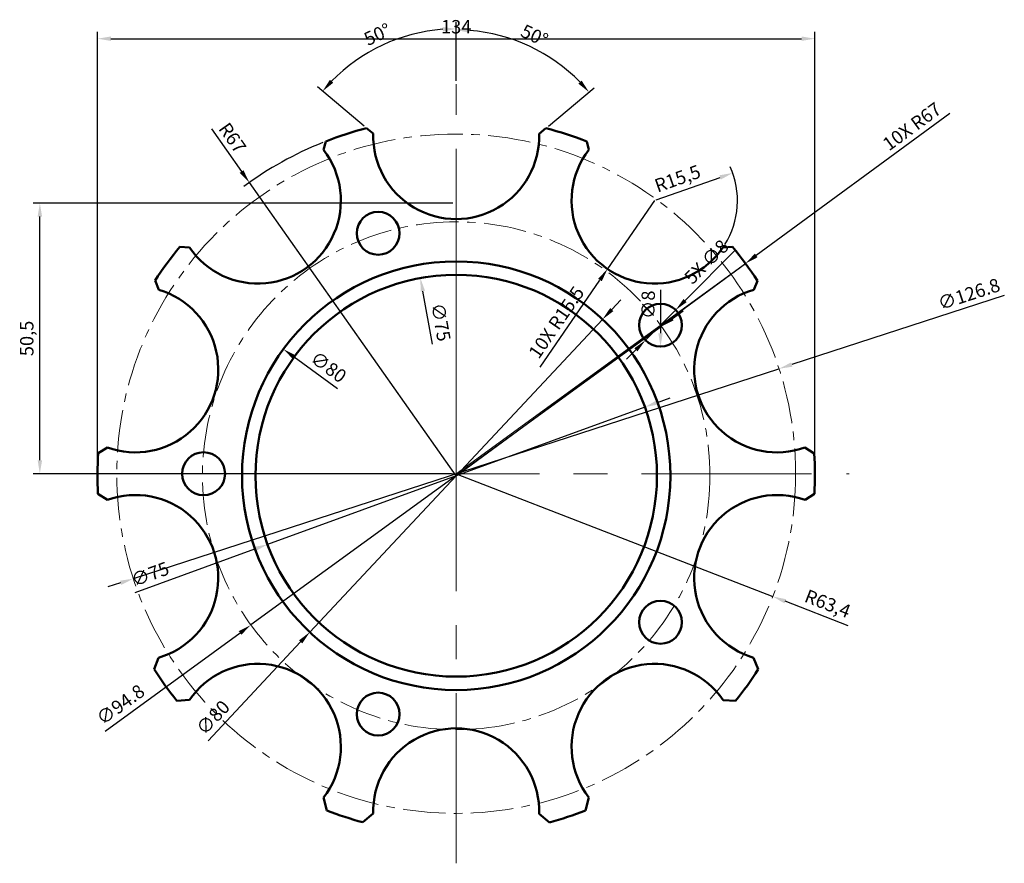
# Model space of a CAD drawing. Units: millimetres. Extents: x 3156 to 3340, y 1440 to 1598.
import ezdxf

# ---------------------------------------------------------------- set-up
doc = ezdxf.new("R2010")
doc.units = ezdxf.units.MM
doc.linetypes.add('CENTER', pattern=[50.8, 31.75, -6.35, 6.35, -6.35])
for name, color, linetype, lineweight in [('M-CNTR', 4, 'CENTER', 18), ('M-CONS', 8, 'Continuous', 13), ('M-DIMS', 2, 'Continuous', 25), ('M-OUTL', 7, 'Continuous', 50)]:
    doc.layers.add(name, color=color, linetype=linetype, lineweight=lineweight)
doc.styles.get("Standard").update_dxf_attribs({"font": 'arial.ttf'})
doc.dimstyles.new('ISO-25', dxfattribs={"dimtxt": 2.5, "dimasz": 2.5, "dimexe": 1.25, "dimexo": 0.625, "dimtad": 1, "dimtxsty": 'Standard', "dimcen": 2.5, "dimadec": 0, "dimazin": 0, "dimtfac": 1, "dimtmove": 0, "dimatfit": 3, "dimfxl": 1, "dimarcsym": 0})

# ---------------------------------------------------------------- blocks, each defined once
blk = doc.blocks.new('*D1')
at = {"layer": 'Defpoints', "color": 0, "transparency": 16777216}
for p in [(3289.21, 1569.14), (3274.59, 1563.99)]:
    blk.add_point(p, dxfattribs=at)
at = {"layer": 'M-DIMS', "color": 0, "lineweight": -2, "transparency": 16777216}
blk.add_line((3274.92, 1564.1), (3286.85, 1568.3), dxfattribs=at)
blk.add_arc((3274.59, 1563.99), 15.5, 327.9019, 24.0231, dxfattribs=at)
at = {"layer": 'M-DIMS', "color": 0, "transparency": 16777216}
blk.add_solid([(3286.71, 1568.7), (3286.99, 1567.91), (3289.21, 1569.14)], dxfattribs=at)
at = {"layer": 'M-DIMS', "color": 0, "transparency": 16777216, "insert": (3279, 1567.79), "char_height": 2.5, "attachment_point": 5, "rotation": 19.4025}
blk.add_mtext('R15,5', dxfattribs=at)
blk = doc.blocks.new('*D2')
at = {"layer": 'Defpoints', "color": 0, "transparency": 16777216}
for p in [(3198.91, 1567.36), (3237.55, 1512.62)]:
    blk.add_point(p, dxfattribs=at)
at = {"layer": 'M-DIMS', "color": 0, "lineweight": -2, "transparency": 16777216}
for p, q in [((3191.86, 1577.35), (3197.47, 1569.4)), ((3237.55, 1512.62), (3198.91, 1567.36))]:
    blk.add_line(p, q, dxfattribs=at)
blk.add_arc((3237.55, 1512.62), 67, 111.8563, 126.2871, dxfattribs=at)
at = {"layer": 'M-DIMS', "color": 0, "transparency": 16777216}
blk.add_solid([(3197.81, 1569.64), (3197.13, 1569.16), (3198.91, 1567.36)], dxfattribs=at)
at = {"layer": 'M-DIMS', "color": 0, "transparency": 16777216, "insert": (3195.5, 1575.49), "char_height": 2.5, "attachment_point": 5, "rotation": 305.2182}
blk.add_mtext('R67', dxfattribs=at)
blk = doc.blocks.new('*D3')
at = {"layer": 'Defpoints', "color": 0, "transparency": 16777216}
for p in [(3237.55, 1513), (3296.66, 1490.09)]:
    blk.add_point(p, dxfattribs=at)
at = {"layer": 'M-DIMS', "color": 0, "lineweight": -2, "transparency": 16777216}
for p, q in [((3237.55, 1513), (3296.66, 1490.09)), ((3310.77, 1484.63), (3299, 1489.19))]:
    blk.add_line(p, q, dxfattribs=at)
at = {"layer": 'M-DIMS', "color": 0, "transparency": 16777216}
blk.add_solid([(3299.15, 1489.58), (3298.85, 1488.8), (3296.66, 1490.09)], dxfattribs=at)
at = {"layer": 'M-DIMS', "color": 0, "transparency": 16777216, "insert": (3306.82, 1488.44), "char_height": 2.5, "attachment_point": 5, "rotation": 338.8209}
blk.add_mtext('R63,4', dxfattribs=at)
blk = doc.blocks.new('*D4')
at = {"layer": 'Defpoints', "color": 0, "transparency": 16777216}
for p in [(3159.78, 1563.5), (3237.55, 1563.5), (3237.28, 1513)]:
    blk.add_point(p, dxfattribs=at)
at = {"layer": 'M-DIMS', "color": 0, "lineweight": -2, "transparency": 16777216}
for p, q in [((3236.92, 1563.5), (3158.53, 1563.5)), ((3159.78, 1515.5), (3159.78, 1561)), ((3236.66, 1513), (3158.53, 1513))]:
    blk.add_line(p, q, dxfattribs=at)
at = {"layer": 'M-DIMS', "color": 0, "transparency": 16777216}
for points in [[(3159.37, 1561), (3160.2, 1561), (3159.78, 1563.5)], [(3159.37, 1515.5), (3160.2, 1515.5), (3159.78, 1513)]]:
    blk.add_solid(points, dxfattribs=at)
at = {"layer": 'M-DIMS', "color": 0, "transparency": 16777216, "insert": (3157.66, 1538.25), "char_height": 2.5, "attachment_point": 5, "rotation": 90}
blk.add_mtext('50,5', dxfattribs=at)
blk = doc.blocks.new('*D5')
at = {"layer": 'Defpoints', "color": 0, "transparency": 16777216}
for p in [(3205.26, 1536.24), (3269.83, 1489.01)]:
    blk.add_point(p, dxfattribs=at)
at = {"layer": 'M-DIMS', "color": 0, "lineweight": -2, "transparency": 16777216}
blk.add_line((3215.39, 1528.83), (3207.28, 1534.76), dxfattribs=at)
at = {"layer": 'M-DIMS', "color": 0, "transparency": 16777216}
blk.add_solid([(3207.53, 1535.1), (3207.03, 1534.43), (3205.26, 1536.24)], dxfattribs=at)
at = {"layer": 'M-DIMS', "color": 0, "transparency": 16777216, "insert": (3213.51, 1532.65), "char_height": 2.5, "attachment_point": 5, "rotation": 323.8166}
blk.add_mtext('∅80', dxfattribs=at)
blk = doc.blocks.new('*D6')
at = {"layer": 'Defpoints', "color": 0, "transparency": 16777216}
for p in [(3230.86, 1549.52), (3244.23, 1475.72)]:
    blk.add_point(p, dxfattribs=at)
at = {"layer": 'M-DIMS', "color": 0, "lineweight": -2, "transparency": 16777216}
blk.add_line((3233.1, 1537.15), (3231.31, 1547.06), dxfattribs=at)
at = {"layer": 'M-DIMS', "color": 0, "transparency": 16777216}
blk.add_solid([(3231.72, 1547.14), (3230.9, 1546.99), (3230.86, 1549.52)], dxfattribs=at)
at = {"layer": 'M-DIMS', "color": 0, "transparency": 16777216, "insert": (3234.37, 1541.23), "char_height": 2.5, "attachment_point": 5, "rotation": 280.2707}
blk.add_mtext('∅75', dxfattribs=at)
blk = doc.blocks.new('*D7')
at = {"layer": 'Defpoints', "color": 0, "transparency": 16777216}
for p in [(3275.71, 1544.73), (3275.71, 1536.73)]:
    blk.add_point(p, dxfattribs=at)
at = {"layer": 'M-DIMS', "color": 0, "lineweight": -2, "transparency": 16777216}
blk.add_line((3275.71, 1547.34), (3275.71, 1539.23), dxfattribs=at)
at = {"layer": 'M-DIMS', "color": 0, "transparency": 16777216}
blk.add_solid([(3275.3, 1539.23), (3276.13, 1539.23), (3275.71, 1536.73)], dxfattribs=at)
at = {"layer": 'M-DIMS', "color": 0, "transparency": 16777216, "insert": (3273.74, 1544.54), "char_height": 2.5, "attachment_point": 5, "rotation": 90}
blk.add_mtext('∅8', dxfattribs=at)
blk = doc.blocks.new('*D8')
at = {"layer": 'Defpoints', "color": 0, "transparency": 16777216}
for p in [(3255.34, 1590.49), (3237.55, 1585.72), (3253.04, 1576.45), (3254.29, 1577.5), (3237.55, 1440.28)]:
    blk.add_point(p, dxfattribs=at)
at = {"layer": 'M-DIMS', "color": 0, "lineweight": -2, "transparency": 16777216}
for p, q in [((3237.55, 1586.34), (3237.55, 1597.08)), ((3254.77, 1577.9), (3263.31, 1585.04))]:
    blk.add_line(p, q, dxfattribs=at)
blk.add_arc((3237.55, 1563.5), 32.33, 44.3295, 85.568, dxfattribs=at)
at = {"layer": 'M-DIMS', "color": 0, "transparency": 16777216}
for points in [[(3240.03, 1595.31), (3240.06, 1596.15), (3237.55, 1595.83)], [(3260.98, 1586.37), (3260.36, 1585.81), (3262.35, 1584.23)]]:
    blk.add_solid(points, dxfattribs=at)
at = {"layer": 'M-DIMS', "color": 0, "transparency": 16777216, "insert": (3252.04, 1594.51), "char_height": 2.5, "attachment_point": 5, "rotation": 334.9488}
blk.add_mtext('50°', dxfattribs=at)
blk = doc.blocks.new('*D9')
at = {"layer": 'Defpoints', "color": 0, "transparency": 16777216}
for p in [(3228.2, 1594.67), (3237.55, 1585.72), (3220.82, 1577.5), (3222.05, 1576.47), (3237.55, 1440.28)]:
    blk.add_point(p, dxfattribs=at)
at = {"layer": 'M-DIMS', "color": 0, "lineweight": -2, "transparency": 16777216}
for p, q in [((3237.55, 1586.34), (3237.55, 1597.29)), ((3220.35, 1577.9), (3211.64, 1585.2))]:
    blk.add_line(p, q, dxfattribs=at)
blk.add_arc((3237.55, 1563.5), 32.55, 94.4023, 135.6561, dxfattribs=at)
at = {"layer": 'M-DIMS', "color": 0, "transparency": 16777216}
for points in [[(3235.03, 1596.36), (3235.06, 1595.53), (3237.55, 1596.04)], [(3214.58, 1585.97), (3213.96, 1586.53), (3212.59, 1584.39)]]:
    blk.add_solid(points, dxfattribs=at)
at = {"layer": 'M-DIMS', "color": 0, "transparency": 16777216, "insert": (3222.97, 1594.71), "char_height": 2.5, "attachment_point": 5, "rotation": 25.0292}
blk.add_mtext('50°', dxfattribs=at)
blk = doc.blocks.new('MOUNTING-HOLE-D8')
blk.add_circle((4, 4), 4)
blk = doc.blocks.new('*D11')
at = {"layer": 'Defpoints', "color": 0, "transparency": 16777216}
for p in [(3304.55, 1594.2), (3170.55, 1513), (3304.55, 1513)]:
    blk.add_point(p, dxfattribs=at)
at = {"layer": 'M-DIMS', "color": 0, "lineweight": -2, "transparency": 16777216}
for p, q in [((3170.55, 1513.62), (3170.55, 1595.45)), ((3304.55, 1513.62), (3304.55, 1595.45)), ((3173.05, 1594.2), (3302.05, 1594.2))]:
    blk.add_line(p, q, dxfattribs=at)
at = {"layer": 'M-DIMS', "color": 0, "transparency": 16777216}
for points in [[(3173.05, 1594.61), (3173.05, 1593.78), (3170.55, 1594.2)], [(3302.05, 1594.61), (3302.05, 1593.78), (3304.55, 1594.2)]]:
    blk.add_solid(points, dxfattribs=at)
at = {"layer": 'M-DIMS', "color": 0, "transparency": 16777216, "insert": (3237.55, 1596.1), "char_height": 2.5, "attachment_point": 5}
blk.add_mtext('134', dxfattribs=at)
blk = doc.blocks.new('*D12')
at = {"layer": 'Defpoints', "color": 0, "transparency": 16777216}
for p in [(3291.57, 1552.25), (3237.55, 1512.62)]:
    blk.add_point(p, dxfattribs=at)
at = {"layer": 'M-DIMS', "color": 0, "lineweight": -2, "transparency": 16777216}
for p, q in [((3329.75, 1580.26), (3293.59, 1553.73)), ((3237.55, 1512.62), (3291.57, 1552.25))]:
    blk.add_line(p, q, dxfattribs=at)
at = {"layer": 'M-DIMS', "color": 0, "transparency": 16777216}
blk.add_solid([(3293.34, 1554.07), (3293.83, 1553.39), (3291.57, 1552.25)], dxfattribs=at)
at = {"layer": 'M-DIMS', "color": 0, "transparency": 16777216, "insert": (3322.86, 1577.56), "char_height": 2.5, "attachment_point": 5, "rotation": 36.2625}
blk.add_mtext('10X R67', dxfattribs=at)
blk = doc.blocks.new('*D13')
at = {"layer": 'Defpoints', "color": 0, "transparency": 16777216}
for p in [(3274.59, 1563.99), (3265.81, 1551.21)]:
    blk.add_point(p, dxfattribs=at)
at = {"layer": 'M-DIMS', "color": 0, "lineweight": -2, "transparency": 16777216}
for p, q in [((3274.59, 1563.99), (3265.81, 1551.21)), ((3253.21, 1532.89), (3264.39, 1549.15))]:
    blk.add_line(p, q, dxfattribs=at)
at = {"layer": 'M-DIMS', "color": 0, "transparency": 16777216}
blk.add_solid([(3264.05, 1549.39), (3264.74, 1548.92), (3265.81, 1551.21)], dxfattribs=at)
at = {"layer": 'M-DIMS', "color": 0, "transparency": 16777216, "insert": (3256.53, 1541.07), "char_height": 2.5, "attachment_point": 5, "rotation": 55.4893}
blk.add_mtext('10X R15.5', dxfattribs=at)
blk = doc.blocks.new('*D14')
at = {"layer": 'Defpoints', "color": 0, "transparency": 16777216}
for p in [(3297.84, 1532.59), (3177.25, 1493.41)]:
    blk.add_point(p, dxfattribs=at)
at = {"layer": 'M-DIMS', "color": 0, "lineweight": -2, "transparency": 16777216}
for p, q in [((3339.92, 1546.26), (3300.22, 1533.36)), ((3177.25, 1493.41), (3297.84, 1532.59)), ((3174.87, 1492.63), (3172.49, 1491.86))]:
    blk.add_line(p, q, dxfattribs=at)
at = {"layer": 'M-DIMS', "color": 0, "transparency": 16777216}
for points in [[(3300.09, 1533.76), (3300.35, 1532.97), (3297.84, 1532.59)], [(3174.74, 1493.03), (3175, 1492.24), (3177.25, 1493.41)]]:
    blk.add_solid(points, dxfattribs=at)
at = {"layer": 'M-DIMS', "color": 0, "transparency": 16777216, "insert": (3333.41, 1546.22), "char_height": 2.5, "attachment_point": 5, "rotation": 18.0004}
blk.add_mtext('∅126.8', dxfattribs=at)
blk = doc.blocks.new('*D15')
at = {"layer": 'Defpoints', "color": 0, "transparency": 16777216}
for p in [(3275.89, 1540.48), (3199.2, 1484.76)]:
    blk.add_point(p, dxfattribs=at)
at = {"layer": 'M-DIMS', "color": 0, "lineweight": -2, "transparency": 16777216}
for p, q in [((3277.92, 1541.95), (3279.94, 1543.42)), ((3275.89, 1540.48), (3199.2, 1484.76)), ((3171.96, 1464.97), (3197.18, 1483.29))]:
    blk.add_line(p, q, dxfattribs=at)
at = {"layer": 'M-DIMS', "color": 0, "transparency": 16777216}
for points in [[(3277.67, 1542.29), (3278.16, 1541.62), (3275.89, 1540.48)], [(3196.93, 1483.63), (3197.42, 1482.95), (3199.2, 1484.76)]]:
    blk.add_solid(points, dxfattribs=at)
at = {"layer": 'M-DIMS', "color": 0, "transparency": 16777216, "insert": (3175.03, 1469.64), "char_height": 2.5, "attachment_point": 5, "rotation": 36.0018}
blk.add_mtext('∅94.8', dxfattribs=at)
blk = doc.blocks.new('*D16')
at = {"layer": 'Defpoints', "color": 0, "transparency": 16777216}
for p in [(3264.89, 1541.81), (3210.2, 1483.43)]:
    blk.add_point(p, dxfattribs=at)
at = {"layer": 'M-DIMS', "color": 0, "lineweight": -2, "transparency": 16777216}
for p, q in [((3266.6, 1543.64), (3268.31, 1545.46)), ((3264.89, 1541.81), (3210.2, 1483.43)), ((3191.21, 1463.16), (3208.49, 1481.61))]:
    blk.add_line(p, q, dxfattribs=at)
at = {"layer": 'M-DIMS', "color": 0, "transparency": 16777216}
for points in [[(3266.3, 1543.92), (3266.91, 1543.35), (3264.89, 1541.81)], [(3208.19, 1481.89), (3208.8, 1481.32), (3210.2, 1483.43)]]:
    blk.add_solid(points, dxfattribs=at)
at = {"layer": 'M-DIMS', "color": 0, "transparency": 16777216, "insert": (3192.35, 1467.26), "char_height": 2.5, "attachment_point": 5, "rotation": 46.8696}
blk.add_mtext('∅80', dxfattribs=at)
blk = doc.blocks.new('*D17')
at = {"layer": 'Defpoints', "color": 0, "transparency": 16777216}
for p in [(3272.79, 1525.44), (3202.31, 1499.8)]:
    blk.add_point(p, dxfattribs=at)
at = {"layer": 'M-DIMS', "color": 0, "lineweight": -2, "transparency": 16777216}
for p, q in [((3275.14, 1526.3), (3277.49, 1527.15)), ((3272.79, 1525.44), (3202.31, 1499.8)), ((3177.61, 1490.82), (3199.96, 1498.95))]:
    blk.add_line(p, q, dxfattribs=at)
at = {"layer": 'M-DIMS', "color": 0, "transparency": 16777216}
for points in [[(3274.99, 1526.69), (3275.28, 1525.91), (3272.79, 1525.44)], [(3199.81, 1499.34), (3200.1, 1498.56), (3202.31, 1499.8)]]:
    blk.add_solid(points, dxfattribs=at)
at = {"layer": 'M-DIMS', "color": 0, "transparency": 16777216, "insert": (3180.49, 1493.96), "char_height": 2.5, "attachment_point": 5, "rotation": 19.9909}
blk.add_mtext('∅75', dxfattribs=at)
blk = doc.blocks.new('*D18')
at = {"layer": 'Defpoints', "color": 0, "transparency": 16777216}
for p in [(3278.54, 1543.56), (3272.89, 1537.9)]:
    blk.add_point(p, dxfattribs=at)
at = {"layer": 'M-DIMS', "color": 0, "lineweight": -2, "transparency": 16777216}
for p, q in [((3289.74, 1554.78), (3280.31, 1545.33)), ((3272.89, 1537.9), (3278.54, 1543.56)), ((3271.12, 1536.13), (3269.35, 1534.36))]:
    blk.add_line(p, q, dxfattribs=at)
at = {"layer": 'M-DIMS', "color": 0, "transparency": 16777216}
for points in [[(3280.01, 1545.62), (3280.6, 1545.03), (3278.54, 1543.56)], [(3270.83, 1536.43), (3271.41, 1535.84), (3272.89, 1537.9)]]:
    blk.add_solid(points, dxfattribs=at)
at = {"layer": 'M-DIMS', "color": 0, "transparency": 16777216, "insert": (3284.51, 1552.33), "char_height": 2.5, "attachment_point": 5, "rotation": 45.0326}
blk.add_mtext('5X ∅8', dxfattribs=at)

msp = doc.modelspace()

# ---------------------------------------------------------------- linework, layer by layer
at = {"layer": 'M-CNTR'}
for p, q in [((3237.547, 1440.28), (3237.547, 1585.718)), ((3170.548, 1512.999), (3304.546, 1512.999))]:
    msp.add_line(p, q, dxfattribs=at)
at = {"layer": 'M-CNTR', "ltscale": 0.25, "transparency": 33554534}
for centre, radius in [((3237.547, 1512.999), 63.4), ((3237.547, 1512.623), 47.4)]:
    msp.add_circle(centre, radius, dxfattribs=at)
at = {"layer": 'M-CONS'}
for p, q in [((3237.547, 1512.999), (3237.547, 1563.499)), ((3291.57, 1552.252), (3237.547, 1512.999)), ((3164.623, 1513.012), (3164.601, 1512.999)), ((3164.601, 1512.999), (3164.644, 1512.999)), ((3164.644, 1512.999), (3164.623, 1513.012)), ((3310.45, 1512.999), (3310.931, 1512.999)), ((3310.471, 1512.986), (3310.493, 1512.999))]:
    msp.add_line(p, q, dxfattribs=at)
at = {"layer": 'M-OUTL'}
for p, q in [((3222.054, 1576.473), (3220.824, 1577.502)), ((3253.041, 1576.453), (3254.29, 1577.497)), ((3212.785, 1573.442), (3213.185, 1575.037)), ((3262.321, 1573.457), (3261.928, 1575.029)), ((3187.704, 1555.244), (3185.951, 1555.364)), ((3287.379, 1555.227), (3289.156, 1555.348)), ((3181.987, 1547.343), (3181.306, 1549.036)), ((3293.126, 1547.349), (3293.799, 1549.019)), ((3172.392, 1517.878), (3170.678, 1516.805)), ((3302.683, 1517.872), (3304.418, 1516.784)), ((3172.411, 1508.126), (3170.632, 1509.242)), ((3302.702, 1508.12), (3304.461, 1509.221)), ((3181.968, 1478.65), (3181.108, 1476.516)), ((3293.107, 1478.655), (3293.974, 1476.498)), ((3187.715, 1470.771), (3185.355, 1470.61)), ((3287.39, 1470.755), (3289.725, 1470.594)), ((3212.773, 1452.541), (3213.375, 1450.135)), ((3262.309, 1452.557), (3261.699, 1450.127)), ((3222.053, 1449.545), (3220.119, 1447.929)), ((3253.04, 1449.525), (3254.954, 1447.923))]:
    msp.add_line(p, q, dxfattribs=at)
for radius in [40, 37.5]:
    msp.add_circle((3237.547, 1512.623), radius, dxfattribs=at)
for centre, radius, start, end in [((3237.547, 1512.623), 67, 104.45334, 111.32186), ((3237.547, 1576.023), 15.5, 178.33535, 1.59162), ((3237.547, 1512.623), 67, 68.66056, 75.52904), ((3200.503, 1563.986), 15.5, 214.33535, 37.59162), ((3274.591, 1563.986), 15.5, 142.33535, 325.59162), ((3237.547, 1512.623), 67, 140.36181, 147.07852), ((3237.547, 1512.623), 67, 32.9038, 39.62043), ((3177.608, 1532.474), 15.5, 250.33535, 73.59162), ((3297.486, 1532.474), 15.5, 106.33535, 289.59162), ((3237.547, 1512.623), 67, 176.42133, 182.8919), ((3237.547, 1512.623), 67, 357.09024, 3.56071), ((3177.608, 1493.524), 15.5, 286.33535, 109.59162), ((3297.486, 1493.524), 15.5, 70.33535, 253.59162), ((3200.503, 1462.012), 15.5, 322.33535, 145.59162), ((3274.591, 1462.012), 15.5, 34.33535, 217.59162), ((3237.547, 1512.623), 67, 212.60888, 218.83272), ((3237.547, 1512.623), 67, 321.14922, 327.37297), ((3237.547, 1449.976), 15.5, 358.33535, 181.59162), ((3237.547, 1512.623), 67, 248.85228, 254.92332), ((3237.547, 1512.623), 67, 285.05848, 291.12949)]:
    msp.add_arc(centre, radius, start, end, dxfattribs=at)

# ---------------------------------------------------------------- block references
for p in [(3218.967, 1553.868), (3271.714, 1536.731), (3186.37, 1508.998), (3271.716, 1481.27), (3218.97, 1464.131)]:
    msp.add_blockref('MOUNTING-HOLE-D8', p, dxfattribs=at)

# ---------------------------------------------------------------- dimensions: what is measured, and where the dimension line sits
at = {"layer": 'M-DIMS'}
dim = msp.add_linear_dim(base=(3304.546, 1594.198), p1=(3170.548, 1512.999), p2=(3304.546, 1512.999), dimstyle='ISO-25', override={"dimdec": 0, "dimlfac": 1, "dimrnd": 0, "dimzin": 0, "dimdsep": 46, "dimlunit": 2}, dxfattribs=at)
dim.commit()
dim.dimension.update_dxf_attribs({"geometry": '*D11', "text_midpoint": (3237.547, 1596.1)})
for base, line2, picture, middle in [((3228.202, 1594.674), ((3222.054, 1576.473), (3220.824, 1577.502)), '*D9', (3222.973, 1594.711)), ((3255.344, 1590.487), ((3253.041, 1576.453), (3254.29, 1577.497)), '*D8', (3252.041, 1594.508))]:
    dim = msp.add_angular_dim_2l(base=base, line1=((3237.547, 1440.28), (3237.547, 1585.718)), line2=line2, dimstyle='ISO-25', override={"dimclrd": 0, "dimclre": 0, "dimclrt": 0}, dxfattribs=at)
    dim.commit()
    dim.dimension.update_dxf_attribs({"geometry": picture, "text_midpoint": middle})
dim = msp.add_radius_dim(center=(3237.547, 1512.623), mpoint=(3291.57, 1552.252), text='10X <>', dimstyle='ISO-25', override={"dimdec": 0, "dimlfac": 1, "dimrnd": 0, "dimzin": 0, "dimdsep": 46, "dimlunit": 2}, dxfattribs=at)
dim.commit()
dim.dimension.update_dxf_attribs({"geometry": '*D12', "text_midpoint": (3323.984, 1576.03), "dimtype": 164})
for center, mpoint, picture, middle in [((3237.547, 1512.623), (3198.909, 1567.359), '*D2', (3195.496, 1575.491)), ((3237.547, 1512.999), (3296.665, 1490.094), '*D3', (3306.817, 1488.442))]:
    dim = msp.add_radius_dim(center=center, mpoint=mpoint, dimstyle='ISO-25', override={"dimclrd": 0, "dimclre": 0, "dimclrt": 0}, dxfattribs=at)
    dim.commit()
    dim.dimension.update_dxf_attribs({"geometry": picture, "text_midpoint": middle})
dim = msp.add_radius_dim(center=(3274.591, 1563.986), mpoint=(3289.211, 1569.135), dimstyle='ISO-25', override={"dimclrd": 0, "dimclre": 0, "dimclrt": 0}, dxfattribs=at)
dim.commit()
dim.dimension.update_dxf_attribs({"geometry": '*D1', "text_midpoint": (3279.706, 1565.787), "dimtype": 164})
dim = msp.add_linear_dim(base=(3159.784, 1563.499), p1=(3237.281, 1512.999), p2=(3237.547, 1563.499), angle=90, dimstyle='ISO-25', override={"dimclrd": 0, "dimclre": 0, "dimclrt": 0}, dxfattribs=at)
dim.commit()
dim.dimension.update_dxf_attribs({"geometry": '*D4', "text_midpoint": (3157.657, 1538.249)})
dim = msp.add_radius_dim(center=(3274.591, 1563.986), mpoint=(3265.809, 1551.214), text='10X <>', dimstyle='ISO-25', override={"dimdec": 1, "dimlfac": 1, "dimrnd": 0, "dimzin": 0, "dimdsep": 46, "dimlunit": 2}, dxfattribs=at)
dim.commit()
dim.dimension.update_dxf_attribs({"geometry": '*D13', "text_midpoint": (3256.528, 1541.07)})
dim = msp.add_diameter_dim_2p(p1=(3272.887, 1537.9), p2=(3278.541, 1543.561), text='5X <>', dimstyle='ISO-25', override={"dimdec": 0, "dimlfac": 1, "dimrnd": 0, "dimzin": 0, "dimdsep": 46, "dimlunit": 2}, dxfattribs=at)
dim.commit()
dim.dimension.update_dxf_attribs({"geometry": '*D18', "text_midpoint": (3285.909, 1550.937)})
for p1, p2, override, picture, middle in [((3177.25, 1493.407), (3297.844, 1532.591), {"dimdec": 1, "dimlfac": 1, "dimrnd": 0, "dimzin": 0, "dimdsep": 46, "dimlunit": 2}, '*D14', (3334.022, 1544.346)), ((3244.233, 1475.723), (3230.861, 1549.522), {"dimclrd": 0, "dimclre": 0, "dimclrt": 0}, '*D6', (3232.427, 1540.877)), ((3275.714, 1544.731), (3275.714, 1536.731), {"dimclrd": 0, "dimclre": 0, "dimclrt": 0}, '*D7', (3275.714, 1544.537)), ((3264.893, 1541.815), (3210.201, 1483.431), {"dimdec": 0, "dimlfac": 1, "dimrnd": 0, "dimzin": 0, "dimdsep": 46, "dimlunit": 2}, '*D16', (3193.793, 1465.915)), ((3275.893, 1540.485), (3199.2, 1484.76), {"dimdec": 1, "dimlfac": 1, "dimrnd": 0, "dimzin": 0, "dimdsep": 46, "dimlunit": 2}, '*D15', (3176.193, 1468.043)), ((3269.832, 1489.008), (3205.262, 1536.237), {"dimclrd": 0, "dimclre": 0, "dimclrt": 0}, '*D5', (3212.341, 1531.059)), ((3272.787, 1525.443), (3202.306, 1499.802), {"dimdec": 0, "dimlfac": 1, "dimrnd": 0, "dimzin": 0, "dimdsep": 46, "dimlunit": 2}, '*D17', (3181.162, 1492.11))]:
    dim = msp.add_diameter_dim_2p(p1=p1, p2=p2, dimstyle='ISO-25', override=override, dxfattribs=at)
    dim.commit()
    dim.dimension.update_dxf_attribs({"geometry": picture, "text_midpoint": middle, "dimtype": 163})

doc.saveas('drawing.dxf')
